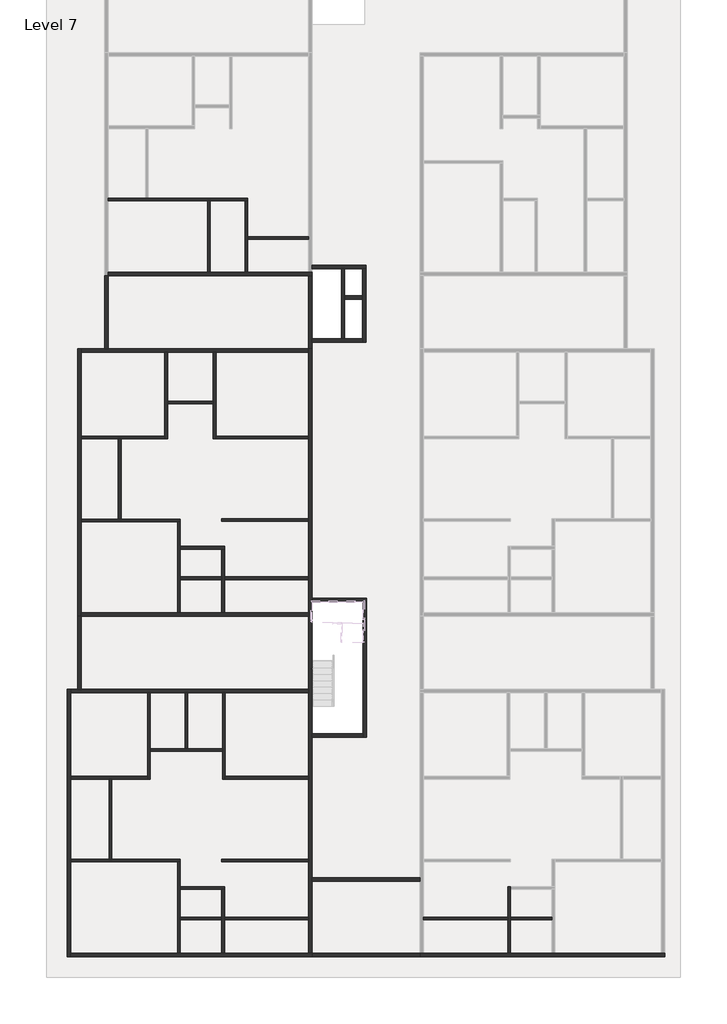
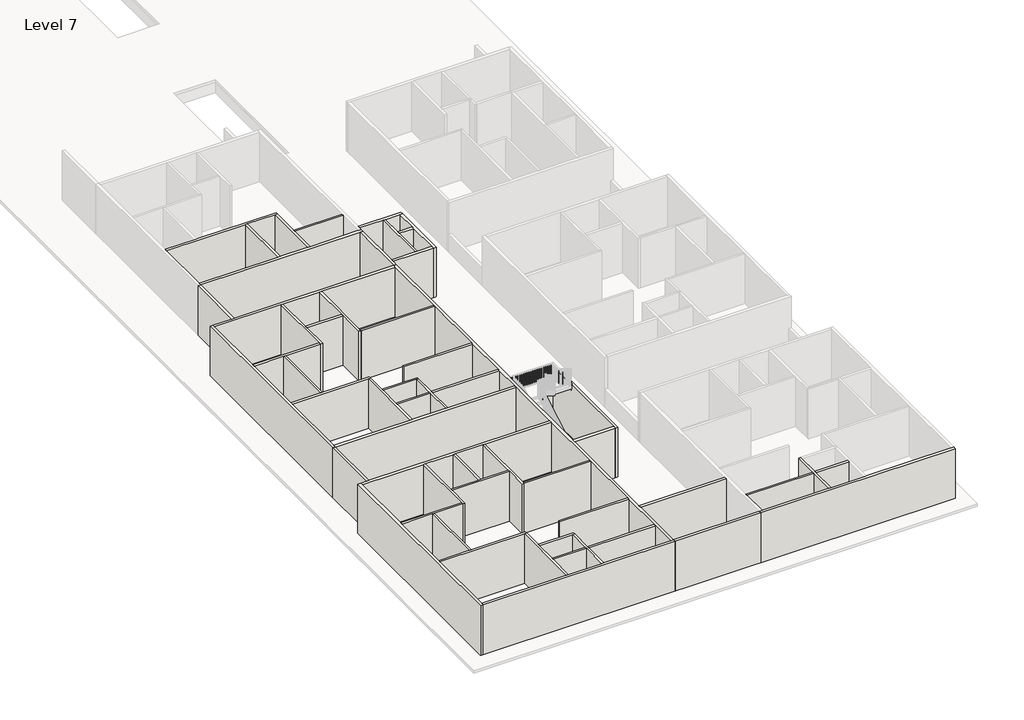
# One storey, part 1 of 8: 55 walls.
"""IFC4 building model written with IfcOpenShell, lengths in millimetres."""

from ifc_helpers import new_model, si_unit, frame, origin, place, context, project, spatial, polyline, outline, extrude, faceted_brep, element, save

model = new_model("IFC4")

# Units and contexts
model_context = context("Model", 3, world=origin())
ifc_project = project(units=[si_unit("LENGTHUNIT", "METRE", prefix="MILLI")], contexts=[model_context])

# Site, building, storey
site = spatial("IfcSite", under=ifc_project)
building = spatial("IfcBuilding", under=site)
storey = spatial("IfcBuildingStorey", under=building, Name="Level 7", Elevation=43522.6172466)

# Walls
placement = place(None, origin())
element("IfcWall", 1, ObjectType="4.5\"", at=placement, inside=storey, context=model_context, shape_type="Brep", body=[
    faceted_brep([(-12531.5544854, -1061.7344126, 43522.6172466), (-8188.1544854, -1061.7344126, 43522.6172466), (-8073.8544854, -1061.7344126, 43522.6172466), (-6549.8544854, -1061.7344126, 43522.6172466), (-6435.5544854, -1061.7344126, 43522.6172466), (-6435.5544854, -1061.7344126, 46570.6172466), (-6549.8544854, -1061.7344126, 46570.6172466), (-8073.8544854, -1061.7344126, 46570.6172466), (-8188.1544854, -1061.7344126, 46570.6172466), (-12531.5544854, -1061.7344126, 46570.6172466), (-12531.5544854, -947.4344126, 43522.6172466), (-12531.5544854, -947.4344126, 46570.6172466), (-10907.2415084, -947.4344126, 46570.6172466), (-10792.9415084, -947.4344126, 46570.6172466), (-6435.5544854, -947.4344126, 46570.6172466), (-6435.5544854, -947.4344126, 43522.6172466), (-10792.9415084, -947.4344126, 43522.6172466), (-10907.2415084, -947.4344126, 43522.6172466)], [[[0, 1, 2, 3, 4, 5, 6, 7, 8, 9]], [[10, 11, 12, 13, 14, 15, 16, 17]], [[4, 3, 2, 1, 0, 10, 17, 16, 15]], [[0, 9, 11, 10]], [[5, 4, 15, 14]], [[9, 8, 7, 6, 5, 14, 13, 12, 11]]]),
])
element("IfcWall", 2, ObjectType="4.5\"", at=placement, inside=storey, context=model_context, shape_type="Brep", body=[
    faceted_brep([(-6549.8544854, -1061.7344126, 43522.6172466), (-6549.8544854, -4185.9344126, 43522.6172466), (-6549.8544854, -4185.9344126, 46570.6172466), (-6549.8544854, -1061.7344126, 46570.6172466), (-6435.5544854, -1061.7344126, 43522.6172466), (-6435.5544854, -1061.7344126, 46570.6172466), (-6435.5544854, -2623.8344126, 46570.6172466), (-6435.5544854, -2738.1344126, 46570.6172466), (-6435.5544854, -4185.9344126, 46570.6172466), (-6435.5544854, -4185.9344126, 43522.6172466), (-6435.5544854, -2738.1344126, 43522.6172466), (-6435.5544854, -2623.8344126, 43522.6172466)], [[[0, 1, 2, 3]], [[4, 5, 6, 7, 8, 9, 10, 11]], [[1, 0, 4, 11, 10, 9]], [[0, 3, 5, 4]], [[2, 1, 9, 8]], [[3, 2, 8, 7, 6, 5]]]),
])
element("IfcWall", 3, ObjectType="4.5\"", at=placement, inside=storey, context=model_context, shape_type="SweptSolid", body=[
    extrude(outline(polyline([(-8188.1544854, -4185.9344126), (-8188.1544854, -1061.7344126), (-8073.8544854, -1061.7344126), (-8073.8544854, -4185.9344126), (-8188.1544854, -4185.9344126)])), frame((0.0, 0.0, 43522.6172466), z_axis=(0.0, 0.0, 1.0), x_axis=(1.0, 0.0, 0.0)), (0.0, 0.0, 1.0), 3048.0),
])
element("IfcWall", 4, ObjectType="4.5\"", at=placement, inside=storey, context=model_context, shape_type="SweptSolid", body=[
    extrude(outline(polyline([(-6435.5544854, -2623.8344126), (-3769.8415084, -2623.8344126), (-3769.8415084, -2738.1344126), (-6435.5544854, -2738.1344126), (-6435.5544854, -2623.8344126)])), frame((0.0, 0.0, 43522.6172466), z_axis=(0.0, 0.0, 1.0), x_axis=(1.0, 0.0, 0.0)), (0.0, 0.0, 1.0), 3048.0),
])
element("IfcWall", 5, ObjectType="4.5\"", at=placement, inside=storey, context=model_context, shape_type="Brep", body=[
    faceted_brep([(-10061.4044854, -7691.1344126, 43522.6172466), (-10061.4044854, -11348.7344126, 43522.6172466), (-10061.4044854, -11463.0344126, 43522.6172466), (-10061.4044854, -11463.0344126, 46570.6172466), (-10061.4044854, -11348.7344126, 46570.6172466), (-10061.4044854, -7691.1344126, 46570.6172466), (-9947.1044854, -7691.1344126, 43522.6172466), (-9947.1044854, -7691.1344126, 46570.6172466), (-9947.1044854, -9824.7344126, 46570.6172466), (-9947.1044854, -9939.0344126, 46570.6172466), (-9947.1044854, -11463.0344126, 46570.6172466), (-9947.1044854, -11463.0344126, 43522.6172466), (-9947.1044854, -9939.0344126, 43522.6172466), (-9947.1044854, -9824.7344126, 43522.6172466)], [[[0, 1, 2, 3, 4, 5]], [[6, 7, 8, 9, 10, 11, 12, 13]], [[2, 1, 0, 6, 13, 12, 11]], [[0, 5, 7, 6]], [[3, 2, 11, 10]], [[5, 4, 3, 10, 9, 8, 7]]]),
])
element("IfcWall", 6, ObjectType="4.5\"", at=placement, inside=storey, context=model_context, shape_type="Brep", body=[
    faceted_brep([(-10061.4044854, -11348.7344126, 43522.6172466), (-13719.0044854, -11348.7344126, 43522.6172466), (-13719.0044854, -11348.7344126, 46570.6172466), (-10061.4044854, -11348.7344126, 46570.6172466), (-10061.4044854, -11463.0344126, 43522.6172466), (-10061.4044854, -11463.0344126, 46570.6172466), (-11980.3915084, -11463.0344126, 46570.6172466), (-12094.6915084, -11463.0344126, 46570.6172466), (-13719.0044854, -11463.0344126, 46570.6172466), (-13719.0044854, -11463.0344126, 43522.6172466), (-12094.6915084, -11463.0344126, 43522.6172466), (-11980.3915084, -11463.0344126, 43522.6172466)], [[[0, 1, 2, 3]], [[4, 5, 6, 7, 8, 9, 10, 11]], [[1, 0, 4, 11, 10, 9]], [[0, 3, 5, 4]], [[2, 1, 9, 8]], [[3, 2, 8, 7, 6, 5]]]),
])
element("IfcWall", 7, ObjectType="4.5\"", at=placement, inside=storey, context=model_context, shape_type="SweptSolid", body=[
    extrude(outline(polyline([(-12094.6915084, -14968.2344126), (-12094.6915084, -11463.0344126), (-11980.3915084, -11463.0344126), (-11980.3915084, -14968.2344126), (-12094.6915084, -14968.2344126)])), frame((0.0, 0.0, 43522.6172466), z_axis=(0.0, 0.0, 1.0), x_axis=(1.0, 0.0, 0.0)), (0.0, 0.0, 1.0), 3048.0),
])
element("IfcWall", 8, ObjectType="4.5\"", at=placement, inside=storey, context=model_context, shape_type="Brep", body=[
    faceted_brep([(-13719.0044854, -15095.2344126, 43522.6172466), (-9510.2415084, -15095.2344126, 43522.6172466), (-9395.9415084, -15095.2344126, 43522.6172466), (-9395.9415084, -15095.2344126, 46570.6172466), (-9510.2415084, -15095.2344126, 46570.6172466), (-13719.0044854, -15095.2344126, 46570.6172466), (-13719.0044854, -14980.9344126, 43522.6172466), (-13719.0044854, -14980.9344126, 46570.6172466), (-9395.9415084, -14980.9344126, 46570.6172466), (-9395.9415084, -14980.9344126, 43522.6172466)], [[[0, 1, 2, 3, 4, 5]], [[6, 7, 8, 9]], [[2, 1, 0, 6, 9]], [[0, 5, 7, 6]], [[3, 2, 9, 8]], [[5, 4, 3, 8, 7]]]),
])
element("IfcWall", 9, ObjectType="4.5\"", at=placement, inside=storey, context=model_context, shape_type="Brep", body=[
    faceted_brep([(-9510.2415084, -15095.2344126, 43522.6172466), (-9510.2415084, -19070.3344126, 43522.6172466), (-9510.2415084, -19070.3344126, 46570.6172466), (-9510.2415084, -15095.2344126, 46570.6172466), (-9395.9415084, -15095.2344126, 43522.6172466), (-9395.9415084, -15095.2344126, 46570.6172466), (-9395.9415084, -16174.7344126, 46570.6172466), (-9395.9415084, -16289.0344126, 46570.6172466), (-9395.9415084, -17508.2344126, 46570.6172466), (-9395.9415084, -17622.5344126, 46570.6172466), (-9395.9415084, -19070.3344126, 46570.6172466), (-9395.9415084, -19070.3344126, 43522.6172466), (-9395.9415084, -17622.5344126, 43522.6172466), (-9395.9415084, -17508.2344126, 43522.6172466), (-9395.9415084, -16289.0344126, 43522.6172466), (-9395.9415084, -16174.7344126, 43522.6172466)], [[[0, 1, 2, 3]], [[4, 5, 6, 7, 8, 9, 10, 11, 12, 13, 14, 15]], [[1, 0, 4, 15, 14, 13, 12, 11]], [[0, 3, 5, 4]], [[2, 1, 11, 10]], [[3, 2, 10, 9, 8, 7, 6, 5]]]),
])
element("IfcWall", 10, ObjectType="4.5\"", at=placement, inside=storey, context=model_context, shape_type="Brep", body=[
    faceted_brep([(-9395.9415084, -16289.0344126, 43522.6172466), (-7567.1415084, -16289.0344126, 43522.6172466), (-7452.8415084, -16289.0344126, 43522.6172466), (-7452.8415084, -16289.0344126, 46570.6172466), (-7567.1415084, -16289.0344126, 46570.6172466), (-9395.9415084, -16289.0344126, 46570.6172466), (-9395.9415084, -16174.7344126, 43522.6172466), (-9395.9415084, -16174.7344126, 46570.6172466), (-7452.8415084, -16174.7344126, 46570.6172466), (-7452.8415084, -16174.7344126, 43522.6172466)], [[[0, 1, 2, 3, 4, 5]], [[6, 7, 8, 9]], [[2, 1, 0, 6, 9]], [[0, 5, 7, 6]], [[3, 2, 9, 8]], [[5, 4, 3, 8, 7]]]),
])
element("IfcWall", 11, ObjectType="4.5\"", at=placement, inside=storey, context=model_context, shape_type="Brep", body=[
    faceted_brep([(-7567.1415084, -16289.0344126, 43522.6172466), (-7567.1415084, -17508.2344126, 43522.6172466), (-7567.1415084, -17622.5344126, 43522.6172466), (-7567.1415084, -19070.3344126, 43522.6172466), (-7567.1415084, -19070.3344126, 46570.6172466), (-7567.1415084, -17622.5344126, 46570.6172466), (-7567.1415084, -17508.2344126, 46570.6172466), (-7567.1415084, -16289.0344126, 46570.6172466), (-7452.8415084, -16289.0344126, 43522.6172466), (-7452.8415084, -16289.0344126, 46570.6172466), (-7452.8415084, -17508.2344126, 46570.6172466), (-7452.8415084, -17622.5344126, 46570.6172466), (-7452.8415084, -19070.3344126, 46570.6172466), (-7452.8415084, -19070.3344126, 43522.6172466), (-7452.8415084, -17622.5344126, 43522.6172466), (-7452.8415084, -17508.2344126, 43522.6172466)], [[[0, 1, 2, 3, 4, 5, 6, 7]], [[8, 9, 10, 11, 12, 13, 14, 15]], [[3, 2, 1, 0, 8, 15, 14, 13]], [[0, 7, 9, 8]], [[4, 3, 13, 12]], [[7, 6, 5, 4, 12, 11, 10, 9]]]),
])
element("IfcWall", 12, ObjectType="4.5\"", at=placement, inside=storey, context=model_context, shape_type="SweptSolid", body=[
    extrude(outline(polyline([(-7567.1415084, -17622.5344126), (-9395.9415084, -17622.5344126), (-9395.9415084, -17508.2344126), (-7567.1415084, -17508.2344126), (-7567.1415084, -17622.5344126)])), frame((0.0, 0.0, 43522.6172466), z_axis=(0.0, 0.0, 1.0), x_axis=(1.0, 0.0, 0.0)), (0.0, 0.0, 1.0), 3048.0),
])
element("IfcWall", 13, ObjectType="4.5\"", at=placement, inside=storey, context=model_context, shape_type="SweptSolid", body=[
    extrude(outline(polyline([(-3769.8415084, -17622.5344126), (-7452.8415084, -17622.5344126), (-7452.8415084, -17508.2344126), (-3769.8415084, -17508.2344126), (-3769.8415084, -17622.5344126)])), frame((0.0, 0.0, 43522.6172466), z_axis=(0.0, 0.0, 1.0), x_axis=(1.0, 0.0, 0.0)), (0.0, 0.0, 1.0), 3048.0),
])
element("IfcWall", 14, ObjectType="4.5\"", at=placement, inside=storey, context=model_context, shape_type="SweptSolid", body=[
    extrude(outline(polyline([(-7567.1415084, -14968.2344126), (-3769.8415084, -14968.2344126), (-3769.8415084, -15082.5344126), (-7567.1415084, -15082.5344126), (-7567.1415084, -14968.2344126)])), frame((0.0, 0.0, 43522.6172466), z_axis=(0.0, 0.0, 1.0), x_axis=(1.0, 0.0, 0.0)), (0.0, 0.0, 1.0), 3048.0),
])
element("IfcWall", 15, ObjectType="4.5\"", at=placement, inside=storey, context=model_context, shape_type="SweptSolid", body=[
    extrude(outline(polyline([(-7940.5044854, -9939.0344126), (-9947.1044854, -9939.0344126), (-9947.1044854, -9824.7344126), (-7940.5044854, -9824.7344126), (-7940.5044854, -9939.0344126)])), frame((0.0, 0.0, 43522.6172466), z_axis=(0.0, 0.0, 1.0), x_axis=(1.0, 0.0, 0.0)), (0.0, 0.0, 1.0), 3048.0),
])
element("IfcWall", 16, ObjectType="4.5\"", at=placement, inside=storey, context=model_context, shape_type="Brep", body=[
    faceted_brep([(-7940.5044854, -7691.1344126, 43522.6172466), (-7940.5044854, -9824.7344126, 43522.6172466), (-7940.5044854, -9939.0344126, 43522.6172466), (-7940.5044854, -11463.0344126, 43522.6172466), (-7940.5044854, -11463.0344126, 46570.6172466), (-7940.5044854, -9939.0344126, 46570.6172466), (-7940.5044854, -9824.7344126, 46570.6172466), (-7940.5044854, -7691.1344126, 46570.6172466), (-7826.2044854, -7691.1344126, 43522.6172466), (-7826.2044854, -7691.1344126, 46570.6172466), (-7826.2044854, -11348.7344126, 46570.6172466), (-7826.2044854, -11463.0344126, 46570.6172466), (-7826.2044854, -11463.0344126, 43522.6172466), (-7826.2044854, -11348.7344126, 43522.6172466)], [[[0, 1, 2, 3, 4, 5, 6, 7]], [[8, 9, 10, 11, 12, 13]], [[3, 2, 1, 0, 8, 13, 12]], [[0, 7, 9, 8]], [[4, 3, 12, 11]], [[7, 6, 5, 4, 11, 10, 9]]]),
])
element("IfcWall", 17, ObjectType="4.5\"", at=placement, inside=storey, context=model_context, shape_type="SweptSolid", body=[
    extrude(outline(polyline([(-3769.8415084, -11463.0344126), (-7826.2044854, -11463.0344126), (-7826.2044854, -11348.7344126), (-3769.8415084, -11348.7344126), (-3769.8415084, -11463.0344126)])), frame((0.0, 0.0, 43522.6172466), z_axis=(0.0, 0.0, 1.0), x_axis=(1.0, 0.0, 0.0)), (0.0, 0.0, 1.0), 3048.0),
])
element("IfcWall", 18, ObjectType="4.5\"", at=placement, inside=storey, context=model_context, shape_type="Brep", body=[
    faceted_brep([(-10818.3415084, -22575.5344126, 43522.6172466), (-10818.3415084, -26233.1344126, 43522.6172466), (-10818.3415084, -26347.4344126, 43522.6172466), (-10818.3415084, -26347.4344126, 46570.6172466), (-10818.3415084, -26233.1344126, 46570.6172466), (-10818.3415084, -22575.5344126, 46570.6172466), (-10704.0415084, -22575.5344126, 43522.6172466), (-10704.0415084, -22575.5344126, 46570.6172466), (-10704.0415084, -25013.9344126, 46570.6172466), (-10704.0415084, -25128.2344126, 46570.6172466), (-10704.0415084, -26347.4344126, 46570.6172466), (-10704.0415084, -26347.4344126, 43522.6172466), (-10704.0415084, -25128.2344126, 43522.6172466), (-10704.0415084, -25013.9344126, 43522.6172466)], [[[0, 1, 2, 3, 4, 5]], [[6, 7, 8, 9, 10, 11, 12, 13]], [[2, 1, 0, 6, 13, 12, 11]], [[0, 5, 7, 6]], [[3, 2, 11, 10]], [[5, 4, 3, 10, 9, 8, 7]]]),
])
element("IfcWall", 19, ObjectType="4.5\"", at=placement, inside=storey, context=model_context, shape_type="Brep", body=[
    faceted_brep([(-10818.3415084, -26233.1344126, 43522.6172466), (-14171.1415084, -26233.1344126, 43522.6172466), (-14171.1415084, -26233.1344126, 46570.6172466), (-10818.3415084, -26233.1344126, 46570.6172466), (-10818.3415084, -26347.4344126, 43522.6172466), (-10818.3415084, -26347.4344126, 46570.6172466), (-12380.4415084, -26347.4344126, 46570.6172466), (-12494.7415084, -26347.4344126, 46570.6172466), (-14171.1415084, -26347.4344126, 46570.6172466), (-14171.1415084, -26347.4344126, 43522.6172466), (-12494.7415084, -26347.4344126, 43522.6172466), (-12380.4415084, -26347.4344126, 43522.6172466)], [[[0, 1, 2, 3]], [[4, 5, 6, 7, 8, 9, 10, 11]], [[1, 0, 4, 11, 10, 9]], [[0, 3, 5, 4]], [[2, 1, 9, 8]], [[3, 2, 8, 7, 6, 5]]]),
])
element("IfcWall", 20, ObjectType="4.5\"", at=placement, inside=storey, context=model_context, shape_type="SweptSolid", body=[
    extrude(outline(polyline([(-9180.0415084, -25013.9344126), (-9180.0415084, -22575.5344126), (-9065.7415084, -22575.5344126), (-9065.7415084, -25013.9344126), (-9180.0415084, -25013.9344126)])), frame((0.0, 0.0, 43522.6172466), z_axis=(0.0, 0.0, 1.0), x_axis=(1.0, 0.0, 0.0)), (0.0, 0.0, 1.0), 3048.0),
])
element("IfcWall", 21, ObjectType="4.5\"", at=placement, inside=storey, context=model_context, shape_type="Brep", body=[
    faceted_brep([(-10704.0415084, -25128.2344126, 43522.6172466), (-7541.7415084, -25128.2344126, 43522.6172466), (-7541.7415084, -25128.2344126, 46570.6172466), (-10704.0415084, -25128.2344126, 46570.6172466), (-10704.0415084, -25013.9344126, 43522.6172466), (-10704.0415084, -25013.9344126, 46570.6172466), (-9180.0415084, -25013.9344126, 46570.6172466), (-9065.7415084, -25013.9344126, 46570.6172466), (-7541.7415084, -25013.9344126, 46570.6172466), (-7541.7415084, -25013.9344126, 43522.6172466), (-9065.7415084, -25013.9344126, 43522.6172466), (-9180.0415084, -25013.9344126, 43522.6172466)], [[[0, 1, 2, 3]], [[4, 5, 6, 7, 8, 9, 10, 11]], [[1, 0, 4, 11, 10, 9]], [[0, 3, 5, 4]], [[2, 1, 9, 8]], [[3, 2, 8, 7, 6, 5]]]),
])
element("IfcWall", 22, ObjectType="4.5\"", at=placement, inside=storey, context=model_context, shape_type="Brep", body=[
    faceted_brep([(-7541.7415084, -22575.5344126, 43522.6172466), (-7541.7415084, -25013.9344126, 43522.6172466), (-7541.7415084, -25128.2344126, 43522.6172466), (-7541.7415084, -26347.4344126, 43522.6172466), (-7541.7415084, -26347.4344126, 46570.6172466), (-7541.7415084, -25128.2344126, 46570.6172466), (-7541.7415084, -25013.9344126, 46570.6172466), (-7541.7415084, -22575.5344126, 46570.6172466), (-7427.4415084, -22575.5344126, 43522.6172466), (-7427.4415084, -22575.5344126, 46570.6172466), (-7427.4415084, -26233.1344126, 46570.6172466), (-7427.4415084, -26347.4344126, 46570.6172466), (-7427.4415084, -26347.4344126, 43522.6172466), (-7427.4415084, -26233.1344126, 43522.6172466)], [[[0, 1, 2, 3, 4, 5, 6, 7]], [[8, 9, 10, 11, 12, 13]], [[3, 2, 1, 0, 8, 13, 12]], [[0, 7, 9, 8]], [[4, 3, 12, 11]], [[7, 6, 5, 4, 11, 10, 9]]]),
])
element("IfcWall", 23, ObjectType="4.5\"", at=placement, inside=storey, context=model_context, shape_type="SweptSolid", body=[
    extrude(outline(polyline([(-3769.8415084, -26347.4344126), (-7427.4415084, -26347.4344126), (-7427.4415084, -26233.1344126), (-3769.8415084, -26233.1344126), (-3769.8415084, -26347.4344126)])), frame((0.0, 0.0, 43522.6172466), z_axis=(0.0, 0.0, 1.0), x_axis=(1.0, 0.0, 0.0)), (0.0, 0.0, 1.0), 3048.0),
])
element("IfcWall", 24, ObjectType="4.5\"", at=placement, inside=storey, context=model_context, shape_type="SweptSolid", body=[
    extrude(outline(polyline([(-12494.7415084, -29852.6344126), (-12494.7415084, -26347.4344126), (-12380.4415084, -26347.4344126), (-12380.4415084, -29852.6344126), (-12494.7415084, -29852.6344126)])), frame((0.0, 0.0, 43522.6172466), z_axis=(0.0, 0.0, 1.0), x_axis=(1.0, 0.0, 0.0)), (0.0, 0.0, 1.0), 3048.0),
])
element("IfcWall", 25, ObjectType="4.5\"", at=placement, inside=storey, context=model_context, shape_type="Brep", body=[
    faceted_brep([(-14171.1415084, -29966.9344126, 43522.6172466), (-9510.2415084, -29966.9344126, 43522.6172466), (-9395.9415084, -29966.9344126, 43522.6172466), (-9395.9415084, -29966.9344126, 46570.6172466), (-9510.2415084, -29966.9344126, 46570.6172466), (-14171.1415084, -29966.9344126, 46570.6172466), (-14171.1415084, -29852.6344126, 43522.6172466), (-14171.1415084, -29852.6344126, 46570.6172466), (-12494.7415084, -29852.6344126, 46570.6172466), (-12380.4415084, -29852.6344126, 46570.6172466), (-9395.9415084, -29852.6344126, 46570.6172466), (-9395.9415084, -29852.6344126, 43522.6172466), (-12380.4415084, -29852.6344126, 43522.6172466), (-12494.7415084, -29852.6344126, 43522.6172466)], [[[0, 1, 2, 3, 4, 5]], [[6, 7, 8, 9, 10, 11, 12, 13]], [[2, 1, 0, 6, 13, 12, 11]], [[0, 5, 7, 6]], [[3, 2, 11, 10]], [[5, 4, 3, 10, 9, 8, 7]]]),
])
element("IfcWall", 26, ObjectType="4.5\"", at=placement, inside=storey, context=model_context, shape_type="Brep", body=[
    faceted_brep([(-9510.2415084, -29966.9344126, 43522.6172466), (-9510.2415084, -33954.7344126, 43522.6172466), (-9510.2415084, -33954.7344126, 46570.6172466), (-9510.2415084, -29966.9344126, 46570.6172466), (-9395.9415084, -29966.9344126, 43522.6172466), (-9395.9415084, -29966.9344126, 46570.6172466), (-9395.9415084, -31059.1344126, 46570.6172466), (-9395.9415084, -31173.4344126, 46570.6172466), (-9395.9415084, -32392.6344126, 46570.6172466), (-9395.9415084, -32506.9344126, 46570.6172466), (-9395.9415084, -33954.7344126, 46570.6172466), (-9395.9415084, -33954.7344126, 43522.6172466), (-9395.9415084, -32506.9344126, 43522.6172466), (-9395.9415084, -32392.6344126, 43522.6172466), (-9395.9415084, -31173.4344126, 43522.6172466), (-9395.9415084, -31059.1344126, 43522.6172466)], [[[0, 1, 2, 3]], [[4, 5, 6, 7, 8, 9, 10, 11, 12, 13, 14, 15]], [[1, 0, 4, 15, 14, 13, 12, 11]], [[0, 3, 5, 4]], [[2, 1, 11, 10]], [[3, 2, 10, 9, 8, 7, 6, 5]]]),
])
element("IfcWall", 27, ObjectType="4.5\"", at=placement, inside=storey, context=model_context, shape_type="Brep", body=[
    faceted_brep([(-9395.9415084, -31173.4344126, 43522.6172466), (-7567.1415084, -31173.4344126, 43522.6172466), (-7452.8415084, -31173.4344126, 43522.6172466), (-7452.8415084, -31173.4344126, 46570.6172466), (-7567.1415084, -31173.4344126, 46570.6172466), (-9395.9415084, -31173.4344126, 46570.6172466), (-9395.9415084, -31059.1344126, 43522.6172466), (-9395.9415084, -31059.1344126, 46570.6172466), (-7452.8415084, -31059.1344126, 46570.6172466), (-7452.8415084, -31059.1344126, 43522.6172466)], [[[0, 1, 2, 3, 4, 5]], [[6, 7, 8, 9]], [[2, 1, 0, 6, 9]], [[0, 5, 7, 6]], [[3, 2, 9, 8]], [[5, 4, 3, 8, 7]]]),
])
element("IfcWall", 28, ObjectType="4.5\"", at=placement, inside=storey, context=model_context, shape_type="Brep", body=[
    faceted_brep([(-7567.1415084, -31173.4344126, 43522.6172466), (-7567.1415084, -32392.6344126, 43522.6172466), (-7567.1415084, -32506.9344126, 43522.6172466), (-7567.1415084, -33954.7344126, 43522.6172466), (-7567.1415084, -33954.7344126, 46570.6172466), (-7567.1415084, -32506.9344126, 46570.6172466), (-7567.1415084, -32392.6344126, 46570.6172466), (-7567.1415084, -31173.4344126, 46570.6172466), (-7452.8415084, -31173.4344126, 43522.6172466), (-7452.8415084, -31173.4344126, 46570.6172466), (-7452.8415084, -32392.6344126, 46570.6172466), (-7452.8415084, -32506.9344126, 46570.6172466), (-7452.8415084, -33954.7344126, 46570.6172466), (-7452.8415084, -33954.7344126, 43522.6172466), (-7452.8415084, -32506.9344126, 43522.6172466), (-7452.8415084, -32392.6344126, 43522.6172466)], [[[0, 1, 2, 3, 4, 5, 6, 7]], [[8, 9, 10, 11, 12, 13, 14, 15]], [[3, 2, 1, 0, 8, 15, 14, 13]], [[0, 7, 9, 8]], [[4, 3, 13, 12]], [[7, 6, 5, 4, 12, 11, 10, 9]]]),
])
element("IfcWall", 29, ObjectType="4.5\"", at=placement, inside=storey, context=model_context, shape_type="SweptSolid", body=[
    extrude(outline(polyline([(-3769.8415084, -32392.6344126), (-3769.8415084, -32506.9344126), (-7452.8415084, -32506.9344126), (-7452.8415084, -32392.6344126), (-3769.8415084, -32392.6344126)])), frame((0.0, 0.0, 43522.6172466), z_axis=(0.0, 0.0, 1.0), x_axis=(1.0, 0.0, 0.0)), (0.0, 0.0, 1.0), 3048.0),
    extrude(outline(polyline([(-9395.9415084, -32506.9344126), (-9395.9415084, -32392.6344126), (-7567.1415084, -32392.6344126), (-7567.1415084, -32506.9344126), (-9395.9415084, -32506.9344126)])), frame((0.0, 0.0, 43522.6172466), z_axis=(0.0, 0.0, 1.0), x_axis=(1.0, 0.0, 0.0)), (0.0, 0.0, 1.0), 3048.0),
])
element("IfcWall", 30, ObjectType="4.5\"", at=placement, inside=storey, context=model_context, shape_type="SweptSolid", body=[
    extrude(outline(polyline([(-7567.1415084, -29852.6344126), (-3769.8415084, -29852.6344126), (-3769.8415084, -29966.9344126), (-7567.1415084, -29966.9344126), (-7567.1415084, -29852.6344126)])), frame((0.0, 0.0, 43522.6172466), z_axis=(0.0, 0.0, 1.0), x_axis=(1.0, 0.0, 0.0)), (0.0, 0.0, 1.0), 3048.0),
])
element("IfcWall", 31, ObjectType="4.5\"", at=placement, inside=storey, context=model_context, shape_type="SweptSolid", body=[
    extrude(outline(polyline([(4942.3584916, -32506.9344126), (1259.3584916, -32506.9344126), (1259.3584916, -32392.6344126), (4942.3584916, -32392.6344126), (4942.3584916, -32506.9344126)])), frame((0.0, 0.0, 43522.6172466), z_axis=(0.0, 0.0, 1.0), x_axis=(1.0, 0.0, 0.0)), (0.0, 0.0, 1.0), 3048.0),
])
element("IfcWall", 32, ObjectType="4.5\"", at=placement, inside=storey, context=model_context, shape_type="Brep", body=[
    faceted_brep([(4942.3584916, -31059.1344126, 43522.6172466), (4942.3584916, -32392.6344126, 43522.6172466), (4942.3584916, -32506.9344126, 43522.6172466), (4942.3584916, -33954.7344126, 43522.6172466), (4942.3584916, -33954.7344126, 46570.6172466), (4942.3584916, -32506.9344126, 46570.6172466), (4942.3584916, -32392.6344126, 46570.6172466), (4942.3584916, -31059.1344126, 46570.6172466), (5056.6584916, -31059.1344126, 43522.6172466), (5056.6584916, -31059.1344126, 46570.6172466), (5056.6584916, -31173.4344126, 46570.6172466), (5056.6584916, -32392.6344126, 46570.6172466), (5056.6584916, -32506.9344126, 46570.6172466), (5056.6584916, -33954.7344126, 46570.6172466), (5056.6584916, -33954.7344126, 43522.6172466), (5056.6584916, -32506.9344126, 43522.6172466), (5056.6584916, -32392.6344126, 43522.6172466), (5056.6584916, -31173.4344126, 43522.6172466)], [[[0, 1, 2, 3, 4, 5, 6, 7]], [[8, 9, 10, 11, 12, 13, 14, 15, 16, 17]], [[3, 2, 1, 0, 8, 17, 16, 15, 14]], [[4, 3, 14, 13]], [[0, 7, 9, 8]], [[7, 6, 5, 4, 13, 12, 11, 10, 9]]]),
])
element("IfcWall", 33, ObjectType="4.5\"", at=placement, inside=storey, context=model_context, shape_type="SweptSolid", body=[
    extrude(outline(polyline([(6885.4584916, -32506.9344126), (5056.6584916, -32506.9344126), (5056.6584916, -32392.6344126), (6885.4584916, -32392.6344126), (6885.4584916, -32506.9344126)])), frame((0.0, 0.0, 43522.6172466), z_axis=(0.0, 0.0, 1.0), x_axis=(1.0, 0.0, 0.0)), (0.0, 0.0, 1.0), 3048.0),
])
element("IfcWall", 34, ObjectType="4.5\"", at=placement, inside=storey, context=model_context, shape_type="Brep", body=[
    faceted_brep([(-2207.6738684, -7082.6751812, 43522.6172466), (-2207.6738684, -5366.3479894, 43522.6172466), (-2207.6738684, -5213.9479894, 43522.6172466), (-2207.6738684, -4034.6751812, 43522.6172466), (-2207.6738684, -4034.6751812, 46570.6172466), (-2207.6738684, -5213.9479894, 46570.6172466), (-2207.6738684, -5366.3479894, 46570.6172466), (-2207.6738684, -7082.6751812, 46570.6172466), (-2321.9738684, -7082.6751812, 43522.6172466), (-2321.9738684, -7082.6751812, 46570.6172466), (-2321.9738684, -4034.6751812, 46570.6172466), (-2321.9738684, -4034.6751812, 43522.6172466)], [[[0, 1, 2, 3, 4, 5, 6, 7]], [[8, 9, 10, 11]], [[3, 2, 1, 0, 8, 11]], [[7, 6, 5, 4, 10, 9]], [[4, 3, 11, 10]], [[0, 7, 9, 8]]]),
])
element("IfcWall", 35, ObjectType="6\"", at=placement, inside=storey, context=model_context, shape_type="Brep", body=[
    faceted_brep([(-12531.5544854, -4338.3344126, 43522.6172466), (-3769.8415084, -4338.3344126, 43522.6172466), (-3617.4415084, -4338.3344126, 43522.6172466), (-3617.4415084, -4338.3344126, 46570.6172466), (-3769.8415084, -4338.3344126, 46570.6172466), (-12531.5544854, -4338.3344126, 46570.6172466), (-12531.5544854, -4185.9344126, 43522.6172466), (-12531.5544854, -4185.9344126, 46570.6172466), (-8188.1544854, -4185.9344126, 46570.6172466), (-8073.8544854, -4185.9344126, 46570.6172466), (-6549.8544854, -4185.9344126, 46570.6172466), (-6435.5544854, -4185.9344126, 46570.6172466), (-3769.8415084, -4185.9344126, 46570.6172466), (-3617.4415084, -4185.9344126, 46570.6172466), (-3617.4415084, -4185.9344126, 43522.6172466), (-3769.8415084, -4185.9344126, 43522.6172466), (-6435.5544854, -4185.9344126, 43522.6172466), (-6549.8544854, -4185.9344126, 43522.6172466), (-8073.8544854, -4185.9344126, 43522.6172466), (-8188.1544854, -4185.9344126, 43522.6172466)], [[[0, 1, 2, 3, 4, 5]], [[6, 7, 8, 9, 10, 11, 12, 13, 14, 15, 16, 17, 18, 19]], [[2, 1, 0, 6, 19, 18, 17, 16, 15, 14]], [[0, 5, 7, 6]], [[3, 2, 14, 13]], [[5, 4, 3, 13, 12, 11, 10, 9, 8, 7]]]),
])
element("IfcWall", 36, ObjectType="6\"", at=placement, inside=storey, context=model_context, shape_type="Brep", body=[
    faceted_brep([(-13871.4044854, -7538.7344126, 43522.6172466), (-13871.4044854, -19222.7344126, 43522.6172466), (-13871.4044854, -19222.7344126, 46570.6172466), (-13871.4044854, -7538.7344126, 46570.6172466), (-13719.0044854, -7538.7344126, 43522.6172466), (-13719.0044854, -7538.7344126, 46570.6172466), (-13719.0044854, -7691.1344126, 46570.6172466), (-13719.0044854, -11348.7344126, 46570.6172466), (-13719.0044854, -11463.0344126, 46570.6172466), (-13719.0044854, -14980.9344126, 46570.6172466), (-13719.0044854, -15095.2344126, 46570.6172466), (-13719.0044854, -19070.3344126, 46570.6172466), (-13719.0044854, -19222.7344126, 46570.6172466), (-13719.0044854, -19222.7344126, 43522.6172466), (-13719.0044854, -19070.3344126, 43522.6172466), (-13719.0044854, -15095.2344126, 43522.6172466), (-13719.0044854, -14980.9344126, 43522.6172466), (-13719.0044854, -11463.0344126, 43522.6172466), (-13719.0044854, -11348.7344126, 43522.6172466), (-13719.0044854, -7691.1344126, 43522.6172466)], [[[0, 1, 2, 3]], [[4, 5, 6, 7, 8, 9, 10, 11, 12, 13, 14, 15, 16, 17, 18, 19]], [[1, 0, 4, 19, 18, 17, 16, 15, 14, 13]], [[2, 1, 13, 12]], [[0, 3, 5, 4]], [[3, 2, 12, 11, 10, 9, 8, 7, 6, 5]]]),
])
element("IfcWall", 37, ObjectType="6\"", at=placement, inside=storey, context=model_context, shape_type="Brep", body=[
    faceted_brep([(-13719.0044854, -19222.7344126, 43522.6172466), (-3769.8415084, -19222.7344126, 43522.6172466), (-3769.8415084, -19222.7344126, 46570.6172466), (-13719.0044854, -19222.7344126, 46570.6172466), (-13719.0044854, -19070.3344126, 43522.6172466), (-13719.0044854, -19070.3344126, 46570.6172466), (-9510.2415084, -19070.3344126, 46570.6172466), (-9395.9415084, -19070.3344126, 46570.6172466), (-7567.1415084, -19070.3344126, 46570.6172466), (-7452.8415084, -19070.3344126, 46570.6172466), (-3769.8415084, -19070.3344126, 46570.6172466), (-3769.8415084, -19070.3344126, 43522.6172466), (-7452.8415084, -19070.3344126, 43522.6172466), (-7567.1415084, -19070.3344126, 43522.6172466), (-9395.9415084, -19070.3344126, 43522.6172466), (-9510.2415084, -19070.3344126, 43522.6172466)], [[[0, 1, 2, 3]], [[4, 5, 6, 7, 8, 9, 10, 11, 12, 13, 14, 15]], [[1, 0, 4, 15, 14, 13, 12, 11]], [[0, 3, 5, 4]], [[2, 1, 11, 10]], [[3, 2, 10, 9, 8, 7, 6, 5]]]),
])
element("IfcWall", 38, ObjectType="6\"", at=placement, inside=storey, context=model_context, shape_type="Brep", body=[
    faceted_brep([(-3617.4415084, -33954.7344126, 43522.6172466), (-3617.4415084, -30820.9325185, 43522.6172466), (-3617.4415084, -30668.5325185, 43522.6172466), (-3617.4415084, -24525.9851539, 43522.6172466), (-3617.4415084, -24373.5851539, 43522.6172466), (-3617.4415084, -18582.3851539, 43522.6172466), (-3617.4415084, -18429.9851539, 43522.6172466), (-3617.4415084, -7538.7344126, 43522.6172466), (-3617.4415084, -7538.7344126, 46570.6172466), (-3617.4415084, -18429.9851539, 46570.6172466), (-3617.4415084, -18582.3851539, 46570.6172466), (-3617.4415084, -24373.5851539, 46570.6172466), (-3617.4415084, -24525.9851539, 46570.6172466), (-3617.4415084, -30668.5325185, 46570.6172466), (-3617.4415084, -30820.9325185, 46570.6172466), (-3617.4415084, -33954.7344126, 46570.6172466), (-3769.8415084, -33954.7344126, 43522.6172466), (-3769.8415084, -33954.7344126, 46570.6172466), (-3769.8415084, -32506.9344126, 46570.6172466), (-3769.8415084, -32392.6344126, 46570.6172466), (-3769.8415084, -29966.9344126, 46570.6172466), (-3769.8415084, -29852.6344126, 46570.6172466), (-3769.8415084, -26347.4344126, 46570.6172466), (-3769.8415084, -26233.1344126, 46570.6172466), (-3769.8415084, -22575.5344126, 46570.6172466), (-3769.8415084, -22423.1344126, 46570.6172466), (-3769.8415084, -19222.7344126, 46570.6172466), (-3769.8415084, -19070.3344126, 46570.6172466), (-3769.8415084, -17622.5344126, 46570.6172466), (-3769.8415084, -17508.2344126, 46570.6172466), (-3769.8415084, -15082.5344126, 46570.6172466), (-3769.8415084, -14968.2344126, 46570.6172466), (-3769.8415084, -11463.0344126, 46570.6172466), (-3769.8415084, -11348.7344126, 46570.6172466), (-3769.8415084, -7691.1344126, 46570.6172466), (-3769.8415084, -7538.7344126, 46570.6172466), (-3769.8415084, -7538.7344126, 43522.6172466), (-3769.8415084, -7691.1344126, 43522.6172466), (-3769.8415084, -11348.7344126, 43522.6172466), (-3769.8415084, -11463.0344126, 43522.6172466), (-3769.8415084, -14968.2344126, 43522.6172466), (-3769.8415084, -15082.5344126, 43522.6172466), (-3769.8415084, -17508.2344126, 43522.6172466), (-3769.8415084, -17622.5344126, 43522.6172466), (-3769.8415084, -19070.3344126, 43522.6172466), (-3769.8415084, -19222.7344126, 43522.6172466), (-3769.8415084, -22423.1344126, 43522.6172466), (-3769.8415084, -22575.5344126, 43522.6172466), (-3769.8415084, -26233.1344126, 43522.6172466), (-3769.8415084, -26347.4344126, 43522.6172466), (-3769.8415084, -29852.6344126, 43522.6172466), (-3769.8415084, -29966.9344126, 43522.6172466), (-3769.8415084, -32392.6344126, 43522.6172466), (-3769.8415084, -32506.9344126, 43522.6172466)], [[[0, 1, 2, 3, 4, 5, 6, 7, 8, 9, 10, 11, 12, 13, 14, 15]], [[16, 17, 18, 19, 20, 21, 22, 23, 24, 25, 26, 27, 28, 29, 30, 31, 32, 33, 34, 35, 36, 37, 38, 39, 40, 41, 42, 43, 44, 45, 46, 47, 48, 49, 50, 51, 52, 53]], [[7, 6, 5, 4, 3, 2, 1, 0, 16, 53, 52, 51, 50, 49, 48, 47, 46, 45, 44, 43, 42, 41, 40, 39, 38, 37, 36]], [[8, 7, 36, 35]], [[0, 15, 17, 16]], [[15, 14, 13, 12, 11, 10, 9, 8, 35, 34, 33, 32, 31, 30, 29, 28, 27, 26, 25, 24, 23, 22, 21, 20, 19, 18, 17]]]),
])
element("IfcWall", 39, ObjectType="6\"", at=placement, inside=storey, context=model_context, shape_type="Brep", body=[
    faceted_brep([(-3769.8415084, -7538.7344126, 43522.6172466), (-12531.5544854, -7538.7344126, 43522.6172466), (-12683.9544854, -7538.7344126, 43522.6172466), (-13719.0044854, -7538.7344126, 43522.6172466), (-13719.0044854, -7538.7344126, 46570.6172466), (-12683.9544854, -7538.7344126, 46570.6172466), (-12531.5544854, -7538.7344126, 46570.6172466), (-3769.8415084, -7538.7344126, 46570.6172466), (-3769.8415084, -7691.1344126, 43522.6172466), (-3769.8415084, -7691.1344126, 46570.6172466), (-7826.2044854, -7691.1344126, 46570.6172466), (-7940.5044854, -7691.1344126, 46570.6172466), (-9947.1044854, -7691.1344126, 46570.6172466), (-10061.4044854, -7691.1344126, 46570.6172466), (-13719.0044854, -7691.1344126, 46570.6172466), (-13719.0044854, -7691.1344126, 43522.6172466), (-10061.4044854, -7691.1344126, 43522.6172466), (-9947.1044854, -7691.1344126, 43522.6172466), (-7940.5044854, -7691.1344126, 43522.6172466), (-7826.2044854, -7691.1344126, 43522.6172466)], [[[0, 1, 2, 3, 4, 5, 6, 7]], [[8, 9, 10, 11, 12, 13, 14, 15, 16, 17, 18, 19]], [[3, 2, 1, 0, 8, 19, 18, 17, 16, 15]], [[0, 7, 9, 8]], [[4, 3, 15, 14]], [[7, 6, 5, 4, 14, 13, 12, 11, 10, 9]]]),
])
element("IfcWall", 40, ObjectType="6\"", at=placement, inside=storey, context=model_context, shape_type="Brep", body=[
    faceted_brep([(-14323.5415084, -22423.1344126, 43522.6172466), (-14323.5415084, -34107.1344126, 43522.6172466), (-14323.5415084, -34107.1344126, 46570.6172466), (-14323.5415084, -22423.1344126, 46570.6172466), (-14171.1415084, -22423.1344126, 43522.6172466), (-14171.1415084, -22423.1344126, 46570.6172466), (-14171.1415084, -22575.5344126, 46570.6172466), (-14171.1415084, -26233.1344126, 46570.6172466), (-14171.1415084, -26347.4344126, 46570.6172466), (-14171.1415084, -29852.6344126, 46570.6172466), (-14171.1415084, -29966.9344126, 46570.6172466), (-14171.1415084, -33954.7344126, 46570.6172466), (-14171.1415084, -34107.1344126, 46570.6172466), (-14171.1415084, -34107.1344126, 43522.6172466), (-14171.1415084, -33954.7344126, 43522.6172466), (-14171.1415084, -29966.9344126, 43522.6172466), (-14171.1415084, -29852.6344126, 43522.6172466), (-14171.1415084, -26347.4344126, 43522.6172466), (-14171.1415084, -26233.1344126, 43522.6172466), (-14171.1415084, -22575.5344126, 43522.6172466)], [[[0, 1, 2, 3]], [[4, 5, 6, 7, 8, 9, 10, 11, 12, 13, 14, 15, 16, 17, 18, 19]], [[1, 0, 4, 19, 18, 17, 16, 15, 14, 13]], [[2, 1, 13, 12]], [[0, 3, 5, 4]], [[3, 2, 12, 11, 10, 9, 8, 7, 6, 5]]]),
])
element("IfcWall", 41, ObjectType="6\"", at=placement, inside=storey, context=model_context, shape_type="Brep", body=[
    faceted_brep([(-14171.1415084, -34107.1344126, 43522.6172466), (-3617.4415084, -34107.1344126, 43522.6172466), (-3617.4415084, -34107.1344126, 46570.6172466), (-14171.1415084, -34107.1344126, 46570.6172466), (-14171.1415084, -33954.7344126, 43522.6172466), (-14171.1415084, -33954.7344126, 46570.6172466), (-9510.2415084, -33954.7344126, 46570.6172466), (-9395.9415084, -33954.7344126, 46570.6172466), (-7567.1415084, -33954.7344126, 46570.6172466), (-7452.8415084, -33954.7344126, 46570.6172466), (-3769.8415084, -33954.7344126, 46570.6172466), (-3617.4415084, -33954.7344126, 46570.6172466), (-3617.4415084, -33954.7344126, 43522.6172466), (-3769.8415084, -33954.7344126, 43522.6172466), (-7452.8415084, -33954.7344126, 43522.6172466), (-7567.1415084, -33954.7344126, 43522.6172466), (-9395.9415084, -33954.7344126, 43522.6172466), (-9510.2415084, -33954.7344126, 43522.6172466)], [[[0, 1, 2, 3]], [[4, 5, 6, 7, 8, 9, 10, 11, 12, 13, 14, 15, 16, 17]], [[1, 0, 4, 17, 16, 15, 14, 13, 12]], [[0, 3, 5, 4]], [[2, 1, 12, 11]], [[3, 2, 11, 10, 9, 8, 7, 6, 5]]]),
])
element("IfcWall", 42, ObjectType="6\"", at=placement, inside=storey, context=model_context, shape_type="Brep", body=[
    faceted_brep([(-3769.8415084, -22423.1344126, 43522.6172466), (-13719.0044854, -22423.1344126, 43522.6172466), (-13871.4044854, -22423.1344126, 43522.6172466), (-14171.1415084, -22423.1344126, 43522.6172466), (-14171.1415084, -22423.1344126, 46570.6172466), (-13871.4044854, -22423.1344126, 46570.6172466), (-13719.0044854, -22423.1344126, 46570.6172466), (-3769.8415084, -22423.1344126, 46570.6172466), (-3769.8415084, -22575.5344126, 43522.6172466), (-3769.8415084, -22575.5344126, 46570.6172466), (-7427.4415084, -22575.5344126, 46570.6172466), (-7541.7415084, -22575.5344126, 46570.6172466), (-9065.7415084, -22575.5344126, 46570.6172466), (-9180.0415084, -22575.5344126, 46570.6172466), (-10704.0415084, -22575.5344126, 46570.6172466), (-10818.3415084, -22575.5344126, 46570.6172466), (-14171.1415084, -22575.5344126, 46570.6172466), (-14171.1415084, -22575.5344126, 43522.6172466), (-10818.3415084, -22575.5344126, 43522.6172466), (-10704.0415084, -22575.5344126, 43522.6172466), (-9180.0415084, -22575.5344126, 43522.6172466), (-9065.7415084, -22575.5344126, 43522.6172466), (-7541.7415084, -22575.5344126, 43522.6172466), (-7427.4415084, -22575.5344126, 43522.6172466)], [[[0, 1, 2, 3, 4, 5, 6, 7]], [[8, 9, 10, 11, 12, 13, 14, 15, 16, 17, 18, 19, 20, 21, 22, 23]], [[3, 2, 1, 0, 8, 23, 22, 21, 20, 19, 18, 17]], [[0, 7, 9, 8]], [[4, 3, 17, 16]], [[7, 6, 5, 4, 16, 15, 14, 13, 12, 11, 10, 9]]]),
])
element("IfcWall", 43, ObjectType="6\"", at=placement, inside=storey, context=model_context, shape_type="Brep", body=[
    faceted_brep([(1106.9584916, -34107.1344126, 43522.6172466), (11813.0584916, -34107.1344126, 43522.6172466), (11813.0584916, -34107.1344126, 46570.6172466), (1106.9584916, -34107.1344126, 46570.6172466), (1106.9584916, -33954.7344126, 43522.6172466), (1106.9584916, -33954.7344126, 46570.6172466), (1259.3584916, -33954.7344126, 46570.6172466), (4942.3584916, -33954.7344126, 46570.6172466), (5056.6584916, -33954.7344126, 46570.6172466), (6885.4584916, -33954.7344126, 46570.6172466), (6999.7584916, -33954.7344126, 46570.6172466), (11660.6584916, -33954.7344126, 46570.6172466), (11813.0584916, -33954.7344126, 46570.6172466), (11813.0584916, -33954.7344126, 43522.6172466), (11660.6584916, -33954.7344126, 43522.6172466), (6999.7584916, -33954.7344126, 43522.6172466), (6885.4584916, -33954.7344126, 43522.6172466), (5056.6584916, -33954.7344126, 43522.6172466), (4942.3584916, -33954.7344126, 43522.6172466), (1259.3584916, -33954.7344126, 43522.6172466)], [[[0, 1, 2, 3]], [[4, 5, 6, 7, 8, 9, 10, 11, 12, 13, 14, 15, 16, 17, 18, 19]], [[1, 0, 4, 19, 18, 17, 16, 15, 14, 13]], [[2, 1, 13, 12]], [[0, 3, 5, 4]], [[3, 2, 12, 11, 10, 9, 8, 7, 6, 5]]]),
])
element("IfcWall", 44, ObjectType="6\"", at=placement, inside=storey, context=model_context, shape_type="Brep", body=[
    faceted_brep([(-3617.4415084, -18582.3851539, 43522.6172466), (-1382.2415084, -18582.3851539, 43522.6172466), (-1229.8415084, -18582.3851539, 43522.6172466), (-1229.8415084, -18582.3851539, 46570.6172466), (-1382.2415084, -18582.3851539, 46570.6172466), (-3617.4415084, -18582.3851539, 46570.6172466), (-3617.4415084, -18429.9851539, 43522.6172466), (-3617.4415084, -18429.9851539, 46570.6172466), (-1229.8415084, -18429.9851539, 46570.6172466), (-1229.8415084, -18429.9851539, 43522.6172466)], [[[0, 1, 2, 3, 4, 5]], [[6, 7, 8, 9]], [[2, 1, 0, 6, 9]], [[5, 4, 3, 8, 7]], [[0, 5, 7, 6]], [[3, 2, 9, 8]]]),
])
element("IfcWall", 45, ObjectType="6\"", at=placement, inside=storey, context=model_context, shape_type="Brep", body=[
    faceted_brep([(-1382.2415084, -18582.3851539, 43522.6172466), (-1382.2415084, -24373.5851539, 43522.6172466), (-1382.2415084, -24525.9851539, 43522.6172466), (-1382.2415084, -24525.9851539, 46570.6172466), (-1382.2415084, -24373.5851539, 46570.6172466), (-1382.2415084, -18582.3851539, 46570.6172466), (-1229.8415084, -18582.3851539, 43522.6172466), (-1229.8415084, -18582.3851539, 46570.6172466), (-1229.8415084, -24525.9851539, 46570.6172466), (-1229.8415084, -24525.9851539, 43522.6172466)], [[[0, 1, 2, 3, 4, 5]], [[6, 7, 8, 9]], [[2, 1, 0, 6, 9]], [[5, 4, 3, 8, 7]], [[0, 5, 7, 6]], [[3, 2, 9, 8]]]),
])
element("IfcWall", 46, ObjectType="6\"", at=placement, inside=storey, context=model_context, shape_type="SweptSolid", body=[
    extrude(outline(polyline([(-3617.4415084, -24373.5851539), (-1382.2415084, -24373.5851539), (-1382.2415084, -24525.9851539), (-3617.4415084, -24525.9851539), (-3617.4415084, -24373.5851539)])), frame((0.0, 0.0, 43522.6172466), z_axis=(0.0, 0.0, 1.0), x_axis=(1.0, 0.0, 0.0)), (0.0, 0.0, 1.0), 3048.0),
])
element("IfcWall", 47, ObjectType="6\"", at=placement, inside=storey, context=model_context, shape_type="Brep", body=[
    faceted_brep([(-3769.8415084, -4338.3344126, 43522.6172466), (-3769.8415084, -7538.7344126, 43522.6172466), (-3769.8415084, -7538.7344126, 46570.6172466), (-3769.8415084, -4338.3344126, 46570.6172466), (-3617.4415084, -4338.3344126, 43522.6172466), (-3617.4415084, -4338.3344126, 46570.6172466), (-3617.4415084, -7082.6751812, 46570.6172466), (-3617.4415084, -7235.0751812, 46570.6172466), (-3617.4415084, -7538.7344126, 46570.6172466), (-3617.4415084, -7538.7344126, 43522.6172466), (-3617.4415084, -7235.0751812, 43522.6172466), (-3617.4415084, -7082.6751812, 43522.6172466)], [[[0, 1, 2, 3]], [[4, 5, 6, 7, 8, 9, 10, 11]], [[1, 0, 4, 11, 10, 9]], [[0, 3, 5, 4]], [[2, 1, 9, 8]], [[3, 2, 8, 7, 6, 5]]]),
])
element("IfcWall", 48, ObjectType="6\"", at=placement, inside=storey, context=model_context, shape_type="Brep", body=[
    faceted_brep([(-3617.4415084, -4034.6751812, 43522.6172466), (-2321.9738684, -4034.6751812, 43522.6172466), (-2207.6738684, -4034.6751812, 43522.6172466), (-1407.6415084, -4034.6751812, 43522.6172466), (-1255.2415084, -4034.6751812, 43522.6172466), (-1255.2415084, -4034.6751812, 46570.6172466), (-1407.6415084, -4034.6751812, 46570.6172466), (-2207.6738684, -4034.6751812, 46570.6172466), (-2321.9738684, -4034.6751812, 46570.6172466), (-3617.4415084, -4034.6751812, 46570.6172466), (-3617.4415084, -3882.2751812, 43522.6172466), (-3617.4415084, -3882.2751812, 46570.6172466), (-1255.2415084, -3882.2751812, 46570.6172466), (-1255.2415084, -3882.2751812, 43522.6172466)], [[[0, 1, 2, 3, 4, 5, 6, 7, 8, 9]], [[10, 11, 12, 13]], [[4, 3, 2, 1, 0, 10, 13]], [[9, 8, 7, 6, 5, 12, 11]], [[0, 9, 11, 10]], [[5, 4, 13, 12]]]),
])
element("IfcWall", 49, ObjectType="6\"", at=placement, inside=storey, context=model_context, shape_type="Brep", body=[
    faceted_brep([(-1407.6415084, -4034.6751812, 43522.6172466), (-1407.6415084, -5213.9479894, 43522.6172466), (-1407.6415084, -5366.3479894, 43522.6172466), (-1407.6415084, -7082.6751812, 43522.6172466), (-1407.6415084, -7235.0751812, 43522.6172466), (-1407.6415084, -7235.0751812, 46570.6172466), (-1407.6415084, -7082.6751812, 46570.6172466), (-1407.6415084, -5366.3479894, 46570.6172466), (-1407.6415084, -5213.9479894, 46570.6172466), (-1407.6415084, -4034.6751812, 46570.6172466), (-1255.2415084, -4034.6751812, 43522.6172466), (-1255.2415084, -4034.6751812, 46570.6172466), (-1255.2415084, -7235.0751812, 46570.6172466), (-1255.2415084, -7235.0751812, 43522.6172466)], [[[0, 1, 2, 3, 4, 5, 6, 7, 8, 9]], [[10, 11, 12, 13]], [[4, 3, 2, 1, 0, 10, 13]], [[9, 8, 7, 6, 5, 12, 11]], [[0, 9, 11, 10]], [[5, 4, 13, 12]]]),
])
element("IfcWall", 50, ObjectType="6\"", at=placement, inside=storey, context=model_context, shape_type="Brep", body=[
    faceted_brep([(-1407.6415084, -7082.6751812, 43522.6172466), (-2207.6738684, -7082.6751812, 43522.6172466), (-2321.9738684, -7082.6751812, 43522.6172466), (-3617.4415084, -7082.6751812, 43522.6172466), (-3617.4415084, -7082.6751812, 46570.6172466), (-2321.9738684, -7082.6751812, 46570.6172466), (-2207.6738684, -7082.6751812, 46570.6172466), (-1407.6415084, -7082.6751812, 46570.6172466), (-1407.6415084, -7235.0751812, 43522.6172466), (-1407.6415084, -7235.0751812, 46570.6172466), (-3617.4415084, -7235.0751812, 46570.6172466), (-3617.4415084, -7235.0751812, 43522.6172466)], [[[0, 1, 2, 3, 4, 5, 6, 7]], [[8, 9, 10, 11]], [[3, 2, 1, 0, 8, 11]], [[7, 6, 5, 4, 10, 9]], [[0, 7, 9, 8]], [[4, 3, 11, 10]]]),
])
element("IfcWall", 51, ObjectType="6\"", at=placement, inside=storey, context=model_context, shape_type="SweptSolid", body=[
    extrude(outline(polyline([(-2207.6738684, -5213.9479894), (-1407.6415084, -5213.9479894), (-1407.6415084, -5366.3479894), (-2207.6738684, -5366.3479894), (-2207.6738684, -5213.9479894)])), frame((0.0, 0.0, 43522.6172466), z_axis=(0.0, 0.0, 1.0), x_axis=(1.0, 0.0, 0.0)), (0.0, 0.0, 1.0), 3048.0),
])
element("IfcWall", 52, ObjectType="6\" 2", at=placement, inside=storey, context=model_context, shape_type="SweptSolid", body=[
    extrude(outline(polyline([(1106.9584916, -34107.1344126), (-3617.4415084, -34107.1344126), (-3617.4415084, -33954.7344126), (1106.9584916, -33954.7344126), (1106.9584916, -34107.1344126)])), frame((0.0, 0.0, 43522.6172466), z_axis=(0.0, 0.0, 1.0), x_axis=(1.0, 0.0, 0.0)), (0.0, 0.0, 1.0), 3048.0),
])
element("IfcWall", 53, ObjectType="6\" 2", at=placement, inside=storey, context=model_context, shape_type="SweptSolid", body=[
    extrude(outline(polyline([(-3617.4415084, -30668.5325185), (1106.9584916, -30668.5325185), (1106.9584916, -30820.9325185), (-3617.4415084, -30820.9325185), (-3617.4415084, -30668.5325185)])), frame((0.0, 0.0, 43522.6172466), z_axis=(0.0, 0.0, 1.0), x_axis=(1.0, 0.0, 0.0)), (0.0, 0.0, 1.0), 3048.0),
])
element("IfcWall", 54, ObjectType="6\" 2", at=placement, inside=storey, context=model_context, shape_type="SweptSolid", body=[
    extrude(outline(polyline([(-13871.4044854, -22423.1344126), (-13871.4044854, -19222.7344126), (-13719.0044854, -19222.7344126), (-13719.0044854, -22423.1344126), (-13871.4044854, -22423.1344126)])), frame((0.0, 0.0, 43522.6172466), z_axis=(0.0, 0.0, 1.0), x_axis=(1.0, 0.0, 0.0)), (0.0, 0.0, 1.0), 3048.0),
])
element("IfcWall", 55, ObjectType="6\" 2", at=placement, inside=storey, context=model_context, shape_type="SweptSolid", body=[
    extrude(outline(polyline([(-12683.9544854, -7538.7344126), (-12683.9544854, -4338.3344126), (-12531.5544854, -4338.3344126), (-12531.5544854, -7538.7344126), (-12683.9544854, -7538.7344126)])), frame((0.0, 0.0, 43522.6172466), z_axis=(0.0, 0.0, 1.0), x_axis=(1.0, 0.0, 0.0)), (0.0, 0.0, 1.0), 3048.0),
])

save(model, "model.ifc")

# Revit data of these elements
# Type "4.5\""
#   Assembly Code = "B2010"
#   Layers, outside or top first: 0' - 4 1/2" "WALLS" (function 1)
# Type "6\""
#   Assembly Code = "B2010"
#   Layers, outside or top first: 0' - 6" "WALLS" (function 1)
# Type "6\" 2"
#   Assembly Code = "B2010"
#   Layers, outside or top first: 0' - 6" "4'" (function 1)
# Elements 1, 2, 3, 4, 5, 6, 7, 8, 9, 10, 11, 12, 13, 14, 15, 16, 17, 18, 19, 20, 21, 22, 23, 24, 25, 26, 27, 28, 29, 30, 31, 32, 33, 34 (IfcWall, "4.5\"")
#   Top Offset = 0' - 0"
#   Base Offset = 0' - 0"
#   Unconnected Height = 10' - 0"
#   wall height = 10' - 0"
#   Phase Created = New Construction
#   Base Constraint = Level 7
#   Materials on its faces: "WALLS"
# Elements 35, 36, 37, 38, 39, 40, 41, 42, 43, 44, 45, 46, 47, 48, 49, 50, 51 (IfcWall, "6\"")
#   Top Offset = 0' - 0"
#   Base Offset = 0' - 0"
#   Unconnected Height = 10' - 0"
#   wall height = 10' - 0"
#   Phase Created = New Construction
#   Base Constraint = Level 7
#   Materials on its faces: "WALLS"
# Elements 52, 53, 54, 55 (IfcWall, "6\" 2")
#   Top Offset = 0' - 0"
#   Base Offset = 0' - 0"
#   Unconnected Height = 10' - 0"
#   wall height = 10' - 0"
#   Phase Created = New Construction
#   Base Constraint = Level 7
#   Materials on its faces: "4'"
# Materials
#   "WALLS": class "Generic", colour RGB 120 120 120, transparency 0, Cost = 0
#   "4'": class "Generic", colour RGB 120 120 120, transparency 0, Cost = 0
